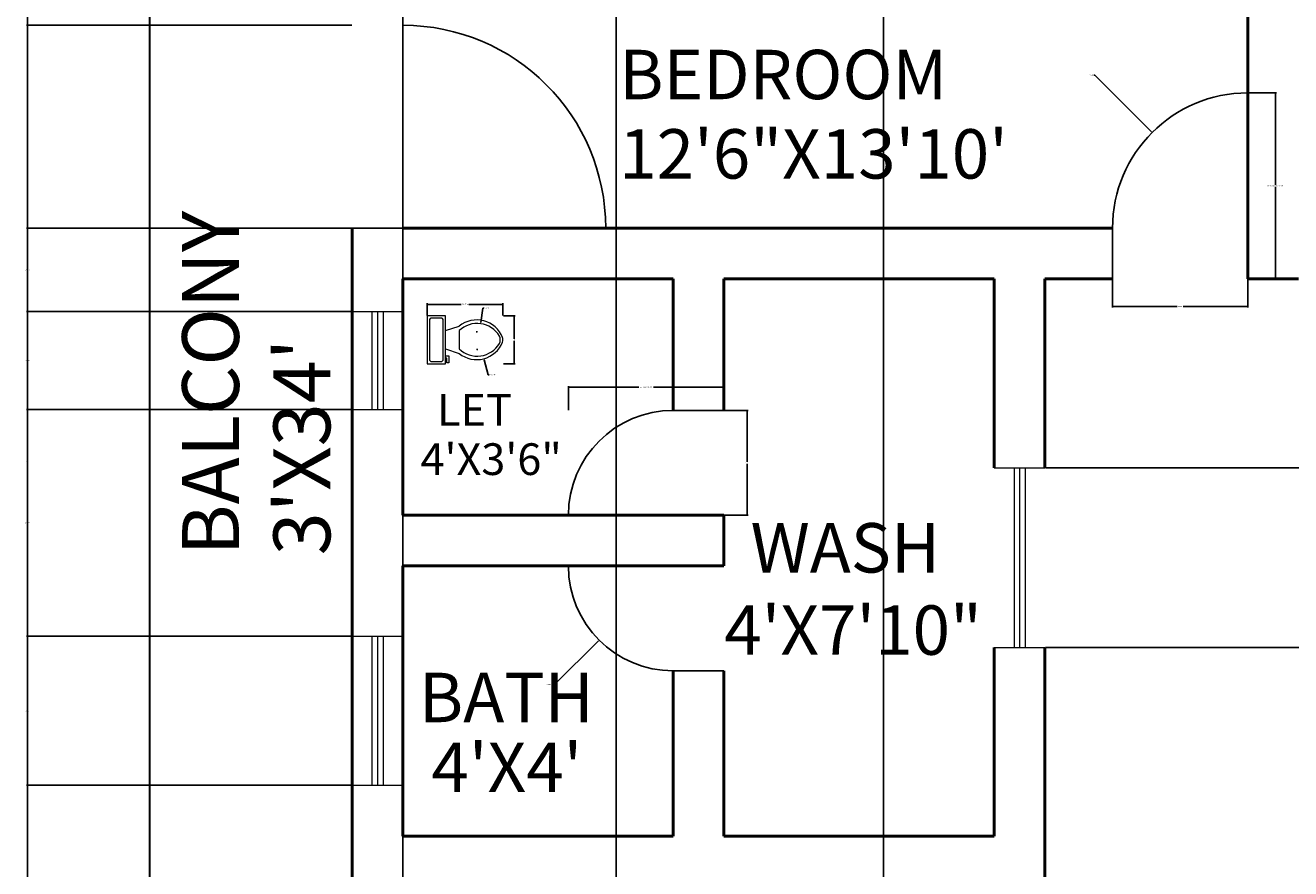
# Model space of a CAD drawing. Units: feet. Extents: x 2387 to 2818, y 1569 to 2046.
# Tile 2 of 4: x 2387 to 2611, y 1735 to 1885. Entities that reach past the tile are written whole.
import ezdxf

# ---------------------------------------------------------------- set-up
doc = ezdxf.new("R2010")
doc.units = ezdxf.units.FT
for name, color, linetype, lineweight in [('A-ANNO-DIMS', 2, 'Continuous', 18), ('A-AREA-IDEN', 7, 'Continuous', 18), ('A-DOOR', 3, 'Continuous', 25), ('A-FLOR-BALC', 7, 'Continuous', 30), ('A-FLOR-FIXT', 9, 'Continuous', 18), ('A-GLAZ', 4, 'Continuous', 18), ('A-WALL', 7, 'Continuous', 50)]:
    doc.layers.add(name, color=color, linetype=linetype, lineweight=lineweight)
doc.styles.get("Standard").update_dxf_attribs({"font": 'arial.ttf'})
doc.dimstyles.get("Standard").update_dxf_attribs({"dimtxt": 0.18, "dimasz": 0.18, "dimexe": 0.18, "dimexo": 0.0625, "dimgap": 0.09, "dimtad": 0, "dimtih": 1, "dimtoh": 1, "dimdec": 4, "dimzin": 0, "dimdsep": 46, "dimtxsty": 'Standard', "dimcen": 0.09, "dimadec": 0, "dimazin": 0, "dimtfac": 1, "dimtdec": 4, "dimtofl": 0, "dimtmove": 0, "dimatfit": 3, "dimfxl": 1, "dimtolj": 1, "dimtzin": 0, "dimarcsym": 0})

# ---------------------------------------------------------------- blocks, each defined once
blk = doc.blocks.new('Toilet - top')
for p, q in [((9.5, -6), (9.5, -2)), ((-10, -8.5), (-8, -8.5)), ((-10, -9.5), (-10, -8.5)), ((-7, -9.5), (-10, -9.5)), ((-8, -8.5), (-8, -8)), ((-7, -8), (-7, -9.5)), ((-4, -8), (-6, -14)), ((4, -8), (6, -14)), ((4, -14), (-4, -14))]:
    blk.add_line(p, q)
blk.add_lwpolyline([(10.5, -8), (10.5, 0), (-10.5, 0), (-10.5, -8)], close=True)
for points in [[(-9.5, -2), (-9.5, -6)], [(8.5, -1), (-8.5, -1)], [(-8.5, -7), (8.5, -7)]]:
    blk.add_lwpolyline(points)
for centre, radius, start, end in [((-8.62, -1.88), 0.884, 81.8699, 188.1301), ((8.62, -1.88), 0.884, 351.8699, 98.1301), ((-8.62, -6.12), 0.884, 171.8699, 278.1301), ((8.62, -6.12), 0.884, 261.8699, 8.1301), ((3.52, -21.58), 12.17, 141.4691, 247.9714), ((4.2, -21.82), 11.33, 136.3677, 238.9468), ((-3.52, -21.58), 12.17, 292.0284, 38.5307), ((-4.2, -21.82), 11.33, 301.053, 43.6321), ((0, -27.88), 4, 245.7318, 294.2682), ((0, -29), 4, 254.8605, 285.1395)]:
    blk.add_arc(centre, radius, start, end)
blk = doc.blocks.new('DOOR-BEDROOM-SWING')
blk.add_line((0, 9), (0, 0))
blk.add_arc((24, 9), 24, 90, 180)
blk = doc.blocks.new('DOOR-BATH-SWING')
blk.add_line((18.62, 0), (27.62, 0))
blk.add_arc((18.62, 18.62), 18.62, 180, 270)
blk = doc.blocks.new('*D17')
at = {"layer": 'A-ANNO-DIMS', "color": 0, "lineweight": -2, "transparency": 16777216}
for p, q in [((2603.8, 1872.82), (2608.87, 1872.82)), ((2608.69, 1872.64), (2608.69, 1856.51)), ((2608.69, 1840), (2608.69, 1856.14)), ((2603.8, 1839.82), (2608.87, 1839.82))]:
    blk.add_line(p, q, dxfattribs=at)
at = {"layer": 'A-ANNO-DIMS', "color": 0, "transparency": 16777216}
for points in [[(2608.66, 1872.64), (2608.72, 1872.64), (2608.69, 1872.82)], [(2608.66, 1840), (2608.72, 1840), (2608.69, 1839.82)]]:
    blk.add_solid(points, dxfattribs=at)
at = {"layer": 'Defpoints', "color": 0, "transparency": 16777216}
for p in [(2603.74, 1872.82), (2608.69, 1872.82), (2603.74, 1839.82)]:
    blk.add_point(p, dxfattribs=at)
at = {"layer": 'A-ANNO-DIMS', "color": 0, "transparency": 16777216, "insert": (2608.69, 1856.32), "char_height": 0.18, "attachment_point": 5}
blk.add_mtext('\\A1;BEDROOM DOOR 33 TYP.', dxfattribs=at)
blk = doc.blocks.new('*D18')
at = {"layer": 'A-ANNO-DIMS', "color": 0, "lineweight": -2, "transparency": 16777216}
for p, q in [((2579.74, 1839.76), (2579.74, 1834.69)), ((2603.74, 1839.76), (2603.74, 1834.69)), ((2579.92, 1834.87), (2591.21, 1834.87)), ((2603.56, 1834.87), (2592.27, 1834.87))]:
    blk.add_line(p, q, dxfattribs=at)
at = {"layer": 'A-ANNO-DIMS', "color": 0, "transparency": 16777216}
for points in [[(2579.92, 1834.9), (2579.92, 1834.84), (2579.74, 1834.87)], [(2603.56, 1834.9), (2603.56, 1834.84), (2603.74, 1834.87)]]:
    blk.add_solid(points, dxfattribs=at)
at = {"layer": 'Defpoints', "color": 0, "transparency": 16777216}
for p in [(2579.74, 1839.82), (2603.74, 1839.82), (2603.74, 1834.87)]:
    blk.add_point(p, dxfattribs=at)
at = {"layer": 'A-ANNO-DIMS', "color": 0, "transparency": 16777216, "insert": (2591.74, 1834.87), "char_height": 0.18, "attachment_point": 5}
blk.add_mtext('\\A1;24 TYP.', dxfattribs=at)
blk = doc.blocks.new('*D19')
at = {"layer": 'A-ANNO-DIMS', "color": 0, "lineweight": -2, "transparency": 16777216}
for p, q in [((2483.12, 1816.51), (2483.12, 1820.77)), ((2483.3, 1820.59), (2495.62, 1820.59)), ((2510.56, 1820.59), (2498.23, 1820.59)), ((2510.74, 1816.51), (2510.74, 1820.77))]:
    blk.add_line(p, q, dxfattribs=at)
at = {"layer": 'A-ANNO-DIMS', "color": 0, "transparency": 16777216}
for points in [[(2483.3, 1820.62), (2483.3, 1820.56), (2483.12, 1820.59)], [(2510.56, 1820.62), (2510.56, 1820.56), (2510.74, 1820.59)]]:
    blk.add_solid(points, dxfattribs=at)
at = {"layer": 'Defpoints', "color": 0, "transparency": 16777216}
for p in [(2510.74, 1820.59), (2483.12, 1816.45), (2510.74, 1816.45)]:
    blk.add_point(p, dxfattribs=at)
at = {"layer": 'A-ANNO-DIMS', "color": 0, "transparency": 16777216, "insert": (2496.93, 1820.59), "char_height": 0.18, "attachment_point": 5}
blk.add_mtext('\\A1;BATH DOOR 28 TYP.', dxfattribs=at)
blk = doc.blocks.new('*D20')
at = {"layer": 'A-ANNO-DIMS', "color": 0, "lineweight": -2, "transparency": 16777216}
for p, q in [((2510.8, 1816.45), (2515.06, 1816.45)), ((2514.88, 1816.27), (2514.88, 1807.32)), ((2514.88, 1798), (2514.88, 1806.95)), ((2510.8, 1797.82), (2515.06, 1797.82))]:
    blk.add_line(p, q, dxfattribs=at)
at = {"layer": 'A-ANNO-DIMS', "color": 0, "transparency": 16777216}
for points in [[(2514.85, 1816.27), (2514.91, 1816.27), (2514.88, 1816.45)], [(2514.85, 1798), (2514.91, 1798), (2514.88, 1797.82)]]:
    blk.add_solid(points, dxfattribs=at)
at = {"layer": 'Defpoints', "color": 0, "transparency": 16777216}
for p in [(2510.74, 1816.45), (2510.74, 1797.82), (2514.88, 1797.82)]:
    blk.add_point(p, dxfattribs=at)
at = {"layer": 'A-ANNO-DIMS', "color": 0, "transparency": 16777216, "insert": (2514.88, 1807.13), "char_height": 0.18, "attachment_point": 5}
blk.add_mtext('\\A1;19 TYP.', dxfattribs=at)
blk = doc.blocks.new('*D25')
at = {"layer": 'A-ANNO-DIMS', "color": 0, "lineweight": -2, "transparency": 16777216}
for p, q in [((2458.04, 1833.32), (2458.04, 1835.46)), ((2458.22, 1835.28), (2464.07, 1835.28)), ((2471.31, 1835.28), (2465.46, 1835.28)), ((2471.49, 1833.32), (2471.49, 1835.46))]:
    blk.add_line(p, q, dxfattribs=at)
at = {"layer": 'A-ANNO-DIMS', "color": 0, "transparency": 16777216}
for points in [[(2458.22, 1835.31), (2458.22, 1835.25), (2458.04, 1835.28)], [(2471.31, 1835.31), (2471.31, 1835.25), (2471.49, 1835.28)]]:
    blk.add_solid(points, dxfattribs=at)
at = {"layer": 'Defpoints', "color": 0, "transparency": 16777216}
for p in [(2458.04, 1835.28), (2458.04, 1833.26), (2471.49, 1833.26)]:
    blk.add_point(p, dxfattribs=at)
at = {"layer": 'A-ANNO-DIMS', "color": 0, "transparency": 16777216, "insert": (2464.77, 1835.28), "char_height": 0.18, "attachment_point": 5}
blk.add_mtext('\\A1;TOILET 13', dxfattribs=at)
blk = doc.blocks.new('*D26')
at = {"layer": 'A-ANNO-DIMS', "color": 0, "lineweight": -2, "transparency": 16777216}
for p, q in [((2471.56, 1833.26), (2473.69, 1833.26)), ((2473.51, 1833.08), (2473.51, 1829.17)), ((2473.51, 1824.89), (2473.51, 1828.8)), ((2471.56, 1824.71), (2473.69, 1824.71))]:
    blk.add_line(p, q, dxfattribs=at)
at = {"layer": 'A-ANNO-DIMS', "color": 0, "transparency": 16777216}
for points in [[(2473.48, 1833.08), (2473.54, 1833.08), (2473.51, 1833.26)], [(2473.48, 1824.89), (2473.54, 1824.89), (2473.51, 1824.71)]]:
    blk.add_solid(points, dxfattribs=at)
at = {"layer": 'Defpoints', "color": 0, "transparency": 16777216}
for p in [(2471.49, 1833.26), (2473.51, 1833.26), (2471.49, 1824.71)]:
    blk.add_point(p, dxfattribs=at)
at = {"layer": 'A-ANNO-DIMS', "color": 0, "transparency": 16777216, "insert": (2473.51, 1828.99), "char_height": 0.18, "attachment_point": 5}
blk.add_mtext('\\A1;9', dxfattribs=at)
blk = doc.blocks.new('*D28')
at = {"layer": 'A-ANNO-DIMS', "color": 0, "lineweight": -2, "transparency": 16777216}
for p, q in [((2408.67, 2023.82), (2386.88, 2023.82)), ((2387.06, 2023.64), (2387.06, 1807.51)), ((2387.06, 1591), (2387.06, 1807.14)), ((2408.67, 1590.82), (2386.88, 1590.82))]:
    blk.add_line(p, q, dxfattribs=at)
at = {"layer": 'A-ANNO-DIMS', "color": 0, "transparency": 16777216}
for points in [[(2387.03, 2023.64), (2387.09, 2023.64), (2387.06, 2023.82)], [(2387.03, 1591), (2387.09, 1591), (2387.06, 1590.82)]]:
    blk.add_solid(points, dxfattribs=at)
at = {"layer": 'Defpoints', "color": 0, "transparency": 16777216}
for p in [(2387.06, 2023.82), (2408.74, 2023.82), (2408.74, 1590.82)]:
    blk.add_point(p, dxfattribs=at)
at = {"layer": 'A-ANNO-DIMS', "color": 0, "transparency": 16777216, "insert": (2387.06, 1807.32), "char_height": 0.18, "attachment_point": 5}
blk.add_mtext('\\A1;433', dxfattribs=at)
blk = doc.blocks.new('*D37')
at = {"layer": 'A-ANNO-DIMS', "color": 0, "lineweight": -2, "transparency": 16777216}
for p, q in [((2491.59, 1599.89), (2491.59, 2045.68)), ((2491.77, 2045.5), (2514.91, 2045.5)), ((2538.86, 2045.5), (2515.71, 2045.5)), ((2539.04, 1599.89), (2539.04, 2045.68))]:
    blk.add_line(p, q, dxfattribs=at)
at = {"layer": 'A-ANNO-DIMS', "color": 0, "transparency": 16777216}
for points in [[(2491.77, 2045.53), (2491.77, 2045.47), (2491.59, 2045.5)], [(2538.86, 2045.53), (2538.86, 2045.47), (2539.04, 2045.5)]]:
    blk.add_solid(points, dxfattribs=at)
at = {"layer": 'Defpoints', "color": 0, "transparency": 16777216}
for p in [(2539.04, 2045.5), (2491.59, 1599.82), (2539.04, 1599.82)]:
    blk.add_point(p, dxfattribs=at)
at = {"layer": 'A-ANNO-DIMS', "color": 0, "transparency": 16777216, "insert": (2515.31, 2045.5), "char_height": 0.18, "attachment_point": 5}
blk.add_mtext('\\A1;47.45', dxfattribs=at)
blk = doc.blocks.new('*D38')
at = {"layer": 'A-ANNO-DIMS', "color": 0, "lineweight": -2, "transparency": 16777216}
for p, q in [((2453.74, 1599.89), (2453.74, 2045.68)), ((2453.92, 2045.5), (2472.27, 2045.5)), ((2491.41, 2045.5), (2473.06, 2045.5)), ((2491.59, 1599.89), (2491.59, 2045.68))]:
    blk.add_line(p, q, dxfattribs=at)
at = {"layer": 'A-ANNO-DIMS', "color": 0, "transparency": 16777216}
for points in [[(2453.92, 2045.53), (2453.92, 2045.47), (2453.74, 2045.5)], [(2491.41, 2045.53), (2491.41, 2045.47), (2491.59, 2045.5)]]:
    blk.add_solid(points, dxfattribs=at)
at = {"layer": 'Defpoints', "color": 0, "transparency": 16777216}
for p in [(2491.59, 2045.5), (2453.74, 1599.82), (2491.59, 1599.82)]:
    blk.add_point(p, dxfattribs=at)
at = {"layer": 'A-ANNO-DIMS', "color": 0, "transparency": 16777216, "insert": (2472.66, 2045.5), "char_height": 0.18, "attachment_point": 5}
blk.add_mtext('\\A1;37.85', dxfattribs=at)
blk = doc.blocks.new('*D41')
at = {"layer": 'A-ANNO-DIMS', "color": 0, "lineweight": -2, "transparency": 16777216}
for p, q in [((2444.67, 1749.91), (2386.88, 1749.91)), ((2387.06, 1749.73), (2387.06, 1717.58)), ((2387.06, 1685.06), (2387.06, 1717.22)), ((2444.67, 1684.88), (2386.88, 1684.88))]:
    blk.add_line(p, q, dxfattribs=at)
at = {"layer": 'A-ANNO-DIMS', "color": 0, "transparency": 16777216}
for points in [[(2387.03, 1749.73), (2387.09, 1749.73), (2387.06, 1749.91)], [(2387.03, 1685.06), (2387.09, 1685.06), (2387.06, 1684.88)]]:
    blk.add_solid(points, dxfattribs=at)
at = {"layer": 'Defpoints', "color": 0, "transparency": 16777216}
for p in [(2387.06, 1749.91), (2444.74, 1749.91), (2444.74, 1684.88)]:
    blk.add_point(p, dxfattribs=at)
at = {"layer": 'A-ANNO-DIMS', "color": 0, "transparency": 16777216, "insert": (2387.06, 1717.4), "char_height": 0.18, "attachment_point": 5}
blk.add_mtext('\\A1;65.03', dxfattribs=at)
blk = doc.blocks.new('*D42')
at = {"layer": 'A-ANNO-DIMS', "color": 0, "lineweight": -2, "transparency": 16777216}
for p, q in [((2444.67, 1776.35), (2386.88, 1776.35)), ((2387.06, 1776.17), (2387.06, 1763.31)), ((2387.06, 1750.09), (2387.06, 1762.95)), ((2444.67, 1749.91), (2386.88, 1749.91))]:
    blk.add_line(p, q, dxfattribs=at)
at = {"layer": 'A-ANNO-DIMS', "color": 0, "transparency": 16777216}
for points in [[(2387.03, 1776.17), (2387.09, 1776.17), (2387.06, 1776.35)], [(2387.03, 1750.09), (2387.09, 1750.09), (2387.06, 1749.91)]]:
    blk.add_solid(points, dxfattribs=at)
at = {"layer": 'Defpoints', "color": 0, "transparency": 16777216}
for p in [(2387.06, 1776.35), (2444.74, 1776.35), (2444.74, 1749.91)]:
    blk.add_point(p, dxfattribs=at)
at = {"layer": 'A-ANNO-DIMS', "color": 0, "transparency": 16777216, "insert": (2387.06, 1763.13), "char_height": 0.18, "attachment_point": 5}
blk.add_mtext('\\A1;26.43', dxfattribs=at)
blk = doc.blocks.new('*D43')
at = {"layer": 'A-ANNO-DIMS', "color": 0, "lineweight": -2, "transparency": 16777216}
for p, q in [((2444.67, 1816.58), (2386.88, 1816.58)), ((2387.06, 1816.4), (2387.06, 1796.64)), ((2387.06, 1776.53), (2387.06, 1796.28)), ((2444.67, 1776.35), (2386.88, 1776.35))]:
    blk.add_line(p, q, dxfattribs=at)
at = {"layer": 'A-ANNO-DIMS', "color": 0, "transparency": 16777216}
for points in [[(2387.03, 1816.4), (2387.09, 1816.4), (2387.06, 1816.58)], [(2387.03, 1776.53), (2387.09, 1776.53), (2387.06, 1776.35)]]:
    blk.add_solid(points, dxfattribs=at)
at = {"layer": 'Defpoints', "color": 0, "transparency": 16777216}
for p in [(2387.06, 1816.58), (2444.74, 1816.58), (2444.74, 1776.35)]:
    blk.add_point(p, dxfattribs=at)
at = {"layer": 'A-ANNO-DIMS', "color": 0, "transparency": 16777216, "insert": (2387.06, 1796.46), "char_height": 0.18, "attachment_point": 5}
blk.add_mtext('\\A1;40.235', dxfattribs=at)
blk = doc.blocks.new('*D44')
at = {"layer": 'A-ANNO-DIMS', "color": 0, "lineweight": -2, "transparency": 16777216}
for p, q in [((2444.67, 1834.03), (2386.88, 1834.03)), ((2387.06, 1833.85), (2387.06, 1825.48)), ((2387.06, 1816.76), (2387.06, 1825.12)), ((2444.67, 1816.58), (2386.88, 1816.58))]:
    blk.add_line(p, q, dxfattribs=at)
at = {"layer": 'A-ANNO-DIMS', "color": 0, "transparency": 16777216}
for points in [[(2387.03, 1833.85), (2387.09, 1833.85), (2387.06, 1834.03)], [(2387.03, 1816.76), (2387.09, 1816.76), (2387.06, 1816.58)]]:
    blk.add_solid(points, dxfattribs=at)
at = {"layer": 'Defpoints', "color": 0, "transparency": 16777216}
for p in [(2387.06, 1834.03), (2444.74, 1834.03), (2444.74, 1816.58)]:
    blk.add_point(p, dxfattribs=at)
at = {"layer": 'A-ANNO-DIMS', "color": 0, "transparency": 16777216, "insert": (2387.06, 1825.3), "char_height": 0.18, "attachment_point": 5}
blk.add_mtext('\\A1;17.447', dxfattribs=at)
blk = doc.blocks.new('*D45')
at = {"layer": 'A-ANNO-DIMS', "color": 0, "lineweight": -2, "transparency": 16777216}
for p, q in [((2444.67, 1848.82), (2386.88, 1848.82)), ((2387.06, 1848.64), (2387.06, 1841.61)), ((2387.06, 1834.21), (2387.06, 1841.24)), ((2444.67, 1834.03), (2386.88, 1834.03))]:
    blk.add_line(p, q, dxfattribs=at)
at = {"layer": 'A-ANNO-DIMS', "color": 0, "transparency": 16777216}
for points in [[(2387.03, 1848.64), (2387.09, 1848.64), (2387.06, 1848.82)], [(2387.03, 1834.21), (2387.09, 1834.21), (2387.06, 1834.03)]]:
    blk.add_solid(points, dxfattribs=at)
at = {"layer": 'Defpoints', "color": 0, "transparency": 16777216}
for p in [(2387.06, 1848.82), (2444.74, 1848.82), (2444.74, 1834.03)]:
    blk.add_point(p, dxfattribs=at)
at = {"layer": 'A-ANNO-DIMS', "color": 0, "transparency": 16777216, "insert": (2387.06, 1841.43), "char_height": 0.18, "attachment_point": 5}
blk.add_mtext('\\A1;14.797', dxfattribs=at)
blk = doc.blocks.new('*D46')
at = {"layer": 'A-ANNO-DIMS', "color": 0, "lineweight": -2, "transparency": 16777216}
for p, q in [((2444.67, 1884.82), (2386.88, 1884.82)), ((2387.06, 1884.64), (2387.06, 1867.01)), ((2387.06, 1849), (2387.06, 1866.64)), ((2444.67, 1848.82), (2386.88, 1848.82))]:
    blk.add_line(p, q, dxfattribs=at)
at = {"layer": 'A-ANNO-DIMS', "color": 0, "transparency": 16777216}
for points in [[(2387.03, 1884.64), (2387.09, 1884.64), (2387.06, 1884.82)], [(2387.03, 1849), (2387.09, 1849), (2387.06, 1848.82)]]:
    blk.add_solid(points, dxfattribs=at)
at = {"layer": 'Defpoints', "color": 0, "transparency": 16777216}
for p in [(2387.06, 1884.82), (2444.74, 1884.82), (2444.74, 1848.82)]:
    blk.add_point(p, dxfattribs=at)
at = {"layer": 'A-ANNO-DIMS', "color": 0, "transparency": 16777216, "insert": (2387.06, 1866.82), "char_height": 0.18, "attachment_point": 5}
blk.add_mtext('\\A1;36', dxfattribs=at)
blk = doc.blocks.new('*D47')
at = {"layer": 'A-ANNO-DIMS', "color": 0, "lineweight": -2, "transparency": 16777216}
for p, q in [((2444.67, 1930.32), (2386.88, 1930.32)), ((2387.06, 1930.14), (2387.06, 1907.76)), ((2387.06, 1885), (2387.06, 1907.39)), ((2444.67, 1884.82), (2386.88, 1884.82))]:
    blk.add_line(p, q, dxfattribs=at)
at = {"layer": 'A-ANNO-DIMS', "color": 0, "transparency": 16777216}
for points in [[(2387.03, 1930.14), (2387.09, 1930.14), (2387.06, 1930.32)], [(2387.03, 1885), (2387.09, 1885), (2387.06, 1884.82)]]:
    blk.add_solid(points, dxfattribs=at)
at = {"layer": 'Defpoints', "color": 0, "transparency": 16777216}
for p in [(2387.06, 1930.32), (2444.74, 1930.32), (2444.74, 1884.82)]:
    blk.add_point(p, dxfattribs=at)
at = {"layer": 'A-ANNO-DIMS', "color": 0, "transparency": 16777216, "insert": (2387.06, 1907.57), "char_height": 0.18, "attachment_point": 5}
blk.add_mtext('\\A1;45.5', dxfattribs=at)
blk = doc.blocks.new('*D62')
at = {"layer": 'A-ANNO-DIMS', "color": 0, "lineweight": -2, "transparency": 16777216}
for p, q in [((2567.8, 1806.26), (2817.6, 1806.26)), ((2817.42, 1806.08), (2817.42, 1790.49)), ((2817.42, 1774.54), (2817.42, 1790.13)), ((2567.8, 1774.36), (2817.6, 1774.36))]:
    blk.add_line(p, q, dxfattribs=at)
at = {"layer": 'A-ANNO-DIMS', "color": 0, "transparency": 16777216}
for points in [[(2817.39, 1806.08), (2817.45, 1806.08), (2817.42, 1806.26)], [(2817.39, 1774.54), (2817.45, 1774.54), (2817.42, 1774.36)]]:
    blk.add_solid(points, dxfattribs=at)
at = {"layer": 'Defpoints', "color": 0, "transparency": 16777216}
for p in [(2567.74, 1806.26), (2817.42, 1806.26), (2567.74, 1774.36)]:
    blk.add_point(p, dxfattribs=at)
at = {"layer": 'A-ANNO-DIMS', "color": 0, "transparency": 16777216, "insert": (2817.42, 1790.31), "char_height": 0.18, "attachment_point": 5}
blk.add_mtext('\\A1;31.904', dxfattribs=at)
blk = doc.blocks.new('*D63')
at = {"layer": 'A-ANNO-DIMS', "color": 0, "lineweight": -2, "transparency": 16777216}
for p, q in [((2567.8, 1774.36), (2817.6, 1774.36)), ((2817.42, 1774.18), (2817.42, 1753.27)), ((2817.42, 1732), (2817.42, 1752.91)), ((2567.8, 1731.82), (2817.6, 1731.82))]:
    blk.add_line(p, q, dxfattribs=at)
at = {"layer": 'A-ANNO-DIMS', "color": 0, "transparency": 16777216}
for points in [[(2817.39, 1774.18), (2817.45, 1774.18), (2817.42, 1774.36)], [(2817.39, 1732), (2817.45, 1732), (2817.42, 1731.82)]]:
    blk.add_solid(points, dxfattribs=at)
at = {"layer": 'Defpoints', "color": 0, "transparency": 16777216}
for p in [(2567.74, 1774.36), (2817.42, 1774.36), (2567.74, 1731.82)]:
    blk.add_point(p, dxfattribs=at)
at = {"layer": 'A-ANNO-DIMS', "color": 0, "transparency": 16777216, "insert": (2817.42, 1753.09), "char_height": 0.18, "attachment_point": 5}
blk.add_mtext('\\A1;42.53', dxfattribs=at)
blk = doc.blocks.new('*D73')
at = {"layer": 'A-ANNO-DIMS', "color": 0, "lineweight": -2, "transparency": 16777216}
for p, q in [((2576.4, 1875.98), (2576.58, 1875.98)), ((2576.58, 1875.98), (2586.64, 1865.92)), ((2603.65, 1848.82), (2603.83, 1848.82)), ((2603.74, 1848.73), (2603.74, 1848.91))]:
    blk.add_line(p, q, dxfattribs=at)
at = {"layer": 'A-ANNO-DIMS', "color": 0, "transparency": 16777216}
blk.add_solid([(2586.66, 1865.94), (2586.62, 1865.9), (2586.77, 1865.79)], dxfattribs=at)
at = {"layer": 'Defpoints', "color": 0, "transparency": 16777216}
for p in [(2586.77, 1865.79), (2603.74, 1848.82)]:
    blk.add_point(p, dxfattribs=at)
at = {"layer": 'A-ANNO-DIMS', "color": 0, "transparency": 16777216, "insert": (2575.9, 1875.98), "char_height": 0.18, "attachment_point": 5}
blk.add_mtext('\\A1;2X R24', dxfattribs=at)
blk = doc.blocks.new('*D75')
at = {"layer": 'A-ANNO-DIMS', "color": 0, "lineweight": -2, "transparency": 16777216}
for p, q in [((2501.65, 1788.82), (2501.83, 1788.82)), ((2501.74, 1788.73), (2501.74, 1788.91)), ((2480.67, 1767.76), (2488.44, 1775.53)), ((2480.49, 1767.76), (2480.67, 1767.76))]:
    blk.add_line(p, q, dxfattribs=at)
at = {"layer": 'A-ANNO-DIMS', "color": 0, "transparency": 16777216}
blk.add_solid([(2488.42, 1775.55), (2488.46, 1775.51), (2488.57, 1775.66)], dxfattribs=at)
at = {"layer": 'Defpoints', "color": 0, "transparency": 16777216}
for p in [(2501.74, 1788.82), (2488.57, 1775.66)]:
    blk.add_point(p, dxfattribs=at)
at = {"layer": 'A-ANNO-DIMS', "color": 0, "transparency": 16777216, "insert": (2479.81, 1767.76), "char_height": 0.18, "attachment_point": 5}
blk.add_mtext('\\A1;2X R18.62', dxfattribs=at)
blk = doc.blocks.new('*D80')
at = {"layer": 'A-ANNO-DIMS', "color": 0, "lineweight": -2, "transparency": 16777216}
for p, q in [((2466.74, 1830.42), (2466.92, 1830.42)), ((2466.83, 1830.33), (2466.83, 1830.51)), ((2468.84, 1822.75), (2468.13, 1825.45)), ((2469.02, 1822.75), (2468.84, 1822.75))]:
    blk.add_line(p, q, dxfattribs=at)
at = {"layer": 'A-ANNO-DIMS', "color": 0, "transparency": 16777216}
blk.add_solid([(2468.16, 1825.46), (2468.1, 1825.45), (2468.08, 1825.63)], dxfattribs=at)
at = {"layer": 'Defpoints', "color": 0, "transparency": 16777216}
for p in [(2466.83, 1830.42), (2468.08, 1825.63)]:
    blk.add_point(p, dxfattribs=at)
at = {"layer": 'A-ANNO-DIMS', "color": 0, "transparency": 16777216, "insert": (2469.69, 1822.75), "char_height": 0.18, "attachment_point": 5}
blk.add_mtext('\\A1;2X R4.953', dxfattribs=at)
blk = doc.blocks.new('*D81')
at = {"layer": 'A-ANNO-DIMS', "color": 0, "lineweight": -2, "transparency": 16777216}
for p, q in [((2467.9, 1834.59), (2467.56, 1832.03)), ((2468.08, 1834.59), (2467.9, 1834.59)), ((2466.83, 1827.28), (2467.01, 1827.28)), ((2466.92, 1827.19), (2466.92, 1827.37))]:
    blk.add_line(p, q, dxfattribs=at)
at = {"layer": 'A-ANNO-DIMS', "color": 0, "transparency": 16777216}
blk.add_solid([(2467.53, 1832.03), (2467.59, 1832.02), (2467.54, 1831.85)], dxfattribs=at)
at = {"layer": 'Defpoints', "color": 0, "transparency": 16777216}
for p in [(2467.54, 1831.85), (2466.92, 1827.28)]:
    blk.add_point(p, dxfattribs=at)
at = {"layer": 'A-ANNO-DIMS', "color": 0, "transparency": 16777216, "insert": (2468.67, 1834.59), "char_height": 0.18, "attachment_point": 5}
blk.add_mtext('\\A1;2X R4.61', dxfattribs=at)

msp = doc.modelspace()

# ---------------------------------------------------------------- linework, layer by layer
at = {"layer": 'A-DOOR'}
for p, q in [((2453.736, 1848.8244), (2444.736, 1848.8244)), ((2501.736, 1788.8244), (2483.736, 1788.8244))]:
    msp.add_line(p, q, dxfattribs=at)
msp.add_arc((2453.736, 1848.8244), 36, 360, 90, dxfattribs=at)
at = {"layer": 'A-FLOR-BALC'}
msp.add_line((2408.736, 2023.8244), (2408.736, 1590.8244), dxfattribs=at)
at = {"layer": 'A-GLAZ'}
for p, q in [((2444.736, 1834.0272), (2453.736, 1834.0272)), ((2448.236, 1834.0272), (2448.236, 1816.58)), ((2449.236, 1834.0272), (2449.236, 1816.58)), ((2450.236, 1834.0272), (2450.236, 1816.58)), ((2444.736, 1816.58), (2453.736, 1816.58)), ((2558.736, 1806.2598), (2567.736, 1806.2598)), ((2562.236, 1806.2598), (2562.236, 1774.356)), ((2563.236, 1806.2598), (2563.236, 1774.356)), ((2564.236, 1806.2598), (2564.236, 1774.356)), ((2444.736, 1776.3453), (2453.736, 1776.3453)), ((2448.236, 1776.3453), (2448.236, 1749.9143)), ((2449.236, 1776.3453), (2449.236, 1749.9143)), ((2450.236, 1776.3453), (2450.236, 1749.9143)), ((2558.736, 1774.356), (2567.736, 1774.356)), ((2444.736, 1749.9143), (2453.736, 1749.9143))]:
    msp.add_line(p, q, dxfattribs=at)
at = {"layer": 'A-WALL'}
for p, q in [((2603.736, 2014.8244), (2603.736, 1839.8244)), ((2444.736, 1590.8244), (2444.736, 1848.8244)), ((2579.736, 1848.8244), (2453.736, 1848.8244)), ((2444.736, 1839.8244), (2444.736, 1797.8244)), ((2453.736, 1839.8244), (2453.736, 1797.8244)), ((2501.736, 1839.8244), (2453.736, 1839.8244)), ((2501.736, 1816.4451), (2501.736, 1839.8244)), ((2510.736, 1816.4451), (2510.736, 1839.8244)), ((2558.736, 1839.8244), (2510.736, 1839.8244)), ((2510.736, 1816.4451), (2510.736, 1839.8244)), ((2558.736, 1806.2598), (2558.736, 1839.8244)), ((2567.736, 1806.2598), (2567.736, 1839.8244)), ((2579.736, 1839.8244), (2567.736, 1839.8244)), ((2612.736, 1839.8244), (2603.736, 1839.8244)), ((2453.736, 1797.8244), (2510.736, 1797.8244)), ((2510.736, 1788.8244), (2510.736, 1797.8244)), ((2444.736, 1788.8244), (2444.736, 1740.8244)), ((2453.736, 1788.8244), (2510.736, 1788.8244)), ((2453.736, 1788.8244), (2453.736, 1740.8244)), ((2558.736, 1740.8244), (2558.736, 1774.356)), ((2567.736, 1731.8244), (2567.736, 1774.356)), ((2501.736, 1740.8244), (2501.736, 1770.2037)), ((2501.736, 1770.2037), (2501.736, 1768.6188)), ((2510.736, 1740.8244), (2510.736, 1770.2037)), ((2453.736, 1740.8244), (2501.736, 1740.8244)), ((2510.736, 1740.8244), (2558.736, 1740.8244))]:
    msp.add_line(p, q, dxfattribs=at)

# ---------------------------------------------------------------- block references
at = {"layer": 'A-DOOR'}
for name, p in [('DOOR-BEDROOM-SWING', (2579.736, 1839.824)), ('DOOR-BATH-SWING', (2483.115, 1770.204))]:
    msp.add_blockref(name, p, dxfattribs=at)
at = {"layer": 'A-DOOR', "extrusion": (0, 0, -1), "zscale": -1, "rotation": 180}
msp.add_blockref('DOOR-BATH-SWING', (-2483.115, 1816.4448), dxfattribs=at)
at = {"layer": 'A-FLOR-FIXT', "xscale": 0.4070471373026423, "yscale": 0.4070471373026423, "zscale": 0.4070471373026423, "rotation": 90}
msp.add_blockref('Toilet - top', (2458.0413, 1828.9863), dxfattribs=at)

# ---------------------------------------------------------------- texts
at = {"layer": 'A-AREA-IDEN'}
for s, height, p in [('BEDROOM', 8.77438, (2492.1359, 1871.7003)), ('12\'6"X13\'10\'', 8.774382, (2492.1359, 1857.6051)), ('LET', 5.62707, (2459.7859, 1813.7382)), ('4\'X3\'6"', 5.62707, (2456.8542, 1804.9783)), ('WASH', 8.77438, (2515.4619, 1787.6577)), ('4\'X7\'10"', 8.77438, (2510.7854, 1773.0536)), ('BATH', 8.77438, (2456.5748, 1761.09)), ("4'X4'", 8.77438, (2458.7881, 1748.6932))]:
    msp.add_text(s, height=height, dxfattribs=at).set_placement(p)
for s, p in [('BALCONY', (2424.6196, 1790.7065)), ("3'X34'", (2440.8349, 1790.7065))]:
    msp.add_text(s, height=10.09409, rotation=90, dxfattribs=at).set_placement(p)

# ---------------------------------------------------------------- dimensions: what is measured, and where the dimension line sits
at = {"layer": 'A-ANNO-DIMS'}
for base, p1, p2, picture, middle in [((2491.5876, 2045.5044), (2453.736, 1599.8244), (2491.5876, 1599.8244), '*D38', (2472.6618, 2045.5044)), ((2539.0379, 2045.5044), (2491.5876, 1599.8244), (2539.0379, 1599.8244), '*D37', (2515.3128, 2045.5044))]:
    dim = msp.add_linear_dim(base=base, p1=p1, p2=p2, dimstyle='Standard', override={"dimdec": 2, "dimlfac": 1, "dimrnd": 0, "dimzin": 0, "dimdsep": 46, "dimlunit": 2}, dxfattribs=at)
    dim.commit()
    dim.dimension.update_dxf_attribs({"geometry": picture, "text_midpoint": middle})
for base, p1, p2, override, picture, middle in [((2387.056, 2023.8244), (2408.736, 1590.8244), (2408.736, 2023.8244), {"dimdec": 0, "dimlfac": 1, "dimrnd": 0, "dimzin": 0, "dimdsep": 46, "dimlunit": 2}, '*D28', (2387.056, 1807.3244)), ((2387.056, 1930.3244), (2444.736, 1884.8244), (2444.736, 1930.3244), {"dimdec": 1, "dimlfac": 1, "dimrnd": 0, "dimzin": 0, "dimdsep": 46, "dimlunit": 2}, '*D47', (2387.056, 1907.5744)), ((2387.056, 1884.8244), (2444.736, 1848.8244), (2444.736, 1884.8244), {"dimdec": 0, "dimlfac": 1, "dimrnd": 0, "dimzin": 0, "dimdsep": 46, "dimlunit": 2}, '*D46', (2387.056, 1866.8244)), ((2387.056, 1848.8244), (2444.736, 1834.0272), (2444.736, 1848.8244), {"dimdec": 3, "dimlfac": 1, "dimrnd": 0, "dimzin": 0, "dimdsep": 46, "dimlunit": 2}, '*D45', (2387.056, 1841.4258)), ((2387.056, 1834.0272), (2444.736, 1816.58), (2444.736, 1834.0272), {"dimdec": 3, "dimlfac": 1, "dimrnd": 0, "dimzin": 0, "dimdsep": 46, "dimlunit": 2}, '*D44', (2387.056, 1825.3036)), ((2473.5104, 1833.2603), (2471.4926, 1824.7123), (2471.4926, 1833.2603), {"dimdec": 0, "dimlfac": 1, "dimrnd": 0, "dimzin": 0, "dimdsep": 46, "dimlunit": 2}, '*D26', (2473.5104, 1828.9863)), ((2387.056, 1816.58), (2444.736, 1776.3453), (2444.736, 1816.58), {"dimdec": 3, "dimlfac": 1, "dimrnd": 0, "dimzin": 0, "dimdsep": 46, "dimlunit": 2}, '*D43', (2387.056, 1796.4626)), ((2817.416, 1806.2598), (2567.736, 1774.356), (2567.736, 1806.2598), {"dimdec": 3, "dimlfac": 1, "dimrnd": 0, "dimzin": 0, "dimdsep": 46, "dimlunit": 2}, '*D62', (2817.416, 1790.3079)), ((2387.056, 1776.3453), (2444.736, 1749.9143), (2444.736, 1776.3453), {"dimdec": 2, "dimlfac": 1, "dimrnd": 0, "dimzin": 0, "dimdsep": 46, "dimlunit": 2}, '*D42', (2387.056, 1763.1298)), ((2817.416, 1774.356), (2567.736, 1731.8244), (2567.736, 1774.356), {"dimdec": 2, "dimlfac": 1, "dimrnd": 0, "dimzin": 0, "dimdsep": 46, "dimlunit": 2}, '*D63', (2817.416, 1753.0902)), ((2387.056, 1749.9143), (2444.736, 1684.8801), (2444.736, 1749.9143), {"dimdec": 2, "dimlfac": 1, "dimrnd": 0, "dimzin": 0, "dimdsep": 46, "dimlunit": 2}, '*D41', (2387.056, 1717.3972))]:
    dim = msp.add_linear_dim(base=base, p1=p1, p2=p2, angle=90, dimstyle='Standard', override=override, dxfattribs=at)
    dim.commit()
    dim.dimension.update_dxf_attribs({"geometry": picture, "text_midpoint": middle})
for center, mpoint, override, picture, middle in [((2603.736, 1848.8244), (2586.7652, 1865.7948), {"dimdec": 0, "dimlfac": 1, "dimrnd": 0, "dimzin": 0, "dimdsep": 46, "dimlunit": 2}, '*D73', (2575.9032, 1875.977)), ((2466.922, 1827.2767), (2467.536, 1831.8472), {"dimdec": 2, "dimlfac": 1, "dimrnd": 0, "dimzin": 0, "dimdsep": 46, "dimlunit": 2}, '*D81', (2468.6719, 1834.5894)), ((2466.8255, 1830.4189), (2468.084, 1825.6281), {"dimdec": 3, "dimlfac": 1, "dimrnd": 0, "dimzin": 0, "dimdsep": 46, "dimlunit": 2}, '*D80', (2469.6938, 1822.7535)), ((2501.736, 1788.8244), (2488.5689, 1775.6579), {"dimdec": 2, "dimlfac": 1, "dimrnd": 0, "dimzin": 0, "dimdsep": 46, "dimlunit": 2}, '*D75', (2479.8148, 1767.7579))]:
    dim = msp.add_radius_dim(center=center, mpoint=mpoint, text='2X <>', dimstyle='Standard', override=override, dxfattribs=at)
    dim.commit()
    dim.dimension.update_dxf_attribs({"geometry": picture, "text_midpoint": middle, "dimtype": 164})
for base, p1, p2, angle, text, picture, middle in [((2608.686, 1872.8244), (2603.736, 1839.8244), (2603.736, 1872.8244), 90, 'BEDROOM DOOR <> TYP.', '*D17', (2608.686, 1856.3244)), ((2458.0413, 1835.278), (2471.4926, 1833.2603), (2458.0413, 1833.2603), 180, 'TOILET <>', '*D25', (2464.767, 1835.278)), ((2514.8791, 1797.8244), (2510.736, 1816.4451), (2510.736, 1797.8244), 270, '<> TYP.', '*D20', (2514.8791, 1807.1348))]:
    dim = msp.add_linear_dim(base=base, p1=p1, p2=p2, angle=angle, text=text, dimstyle='Standard', override={"dimdec": 0, "dimlfac": 1, "dimrnd": 0, "dimzin": 0, "dimdsep": 46, "dimlunit": 2}, dxfattribs=at)
    dim.commit()
    dim.dimension.update_dxf_attribs({"geometry": picture, "text_midpoint": middle})
for base, p1, p2, text, picture, middle in [((2603.736, 1834.8744), (2579.736, 1839.8244), (2603.736, 1839.8244), '<> TYP.', '*D18', (2591.736, 1834.8744)), ((2510.736, 1820.5882), (2483.1152, 1816.4451), (2510.736, 1816.4451), 'BATH DOOR <> TYP.', '*D19', (2496.9256, 1820.5882))]:
    dim = msp.add_linear_dim(base=base, p1=p1, p2=p2, text=text, dimstyle='Standard', override={"dimdec": 0, "dimlfac": 1, "dimrnd": 0, "dimzin": 0, "dimdsep": 46, "dimlunit": 2}, dxfattribs=at)
    dim.commit()
    dim.dimension.update_dxf_attribs({"geometry": picture, "text_midpoint": middle})

doc.saveas('drawing.dxf')
